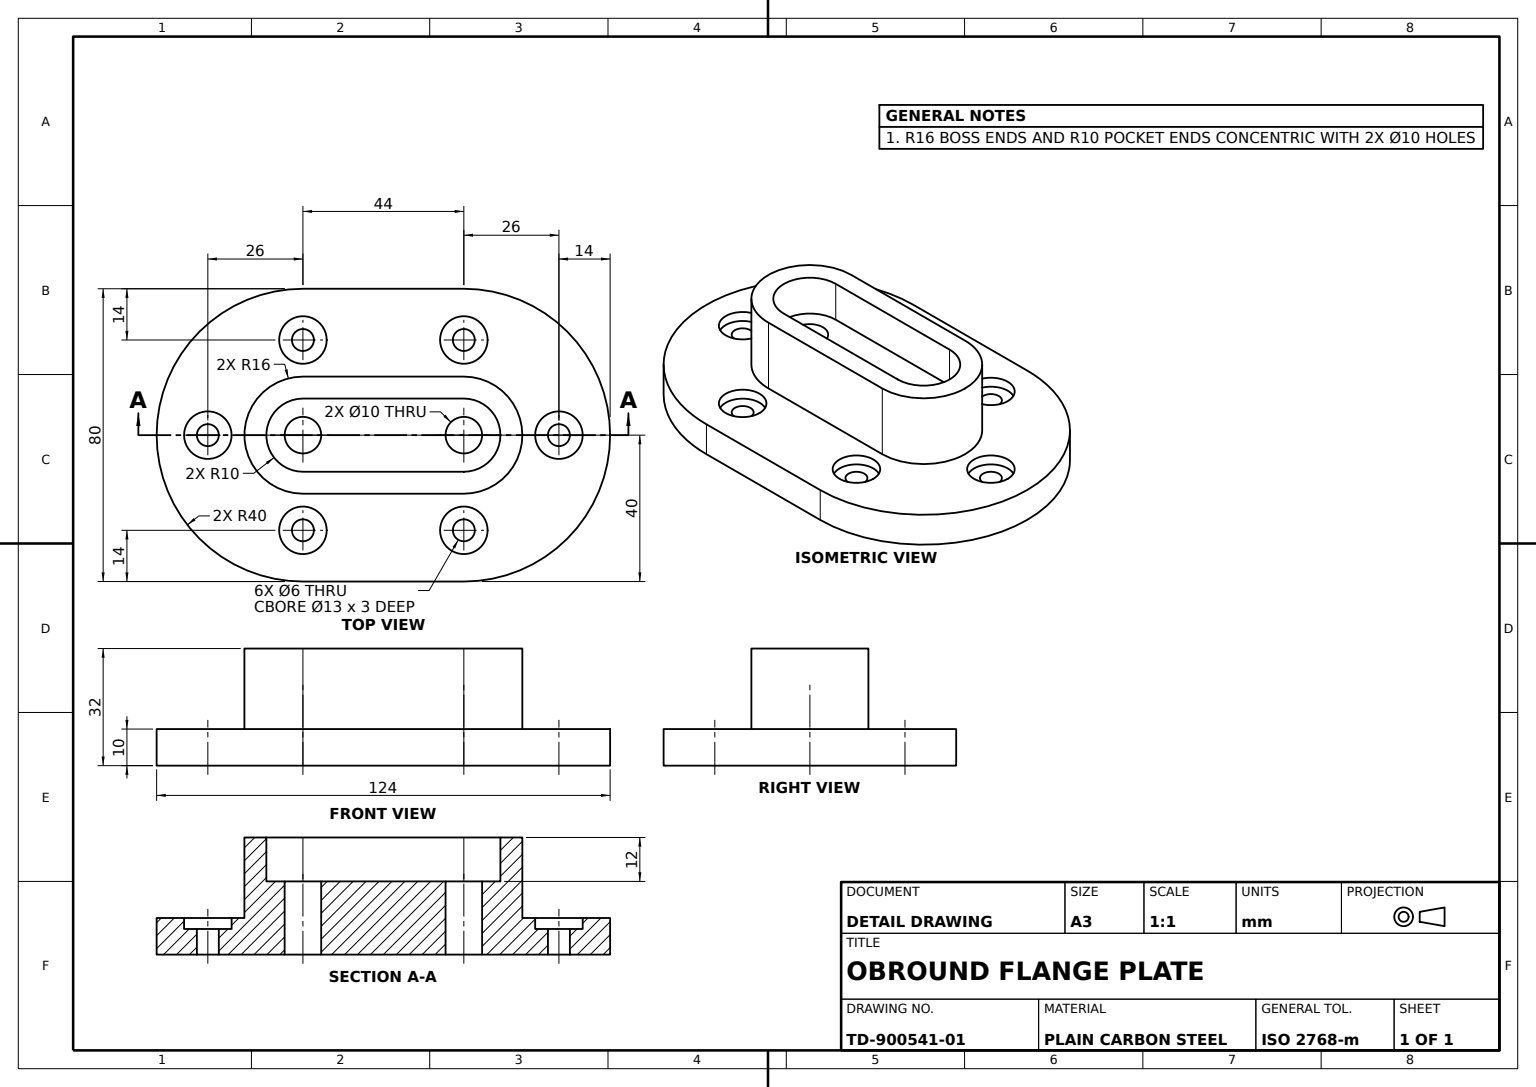
from build123d import *

# Parameters (mm, degrees)
BASE_PLATE_DEPTH        = 10
SLOT_BOSS_DEPTH         = 22
SECONDARY_BOSS_DEPTH    = 10
SLOT_CUT_SKETCH_R       = 5
SLOT_THROUGH_CUT_DEPTH  = 34.5
COUNTERBORE_SKETCH_R    = 6.5
COUNTERBORES_6X_DEPTH   = 3
MOUNTING_HOLE_SKETCH_R  = 3
MOUNTING_HOLES_6X_DEPTH = 88


with BuildPart() as part:
    # Base Plate Sketch → Base Plate (new body)
    with BuildSketch(Plane(origin=(0, 0, 0), x_dir=(1, 0, 0), z_dir=(0, 1, 0))):
        with BuildLine():
            Line((40, 22), (40, -22))
            ThreePointArc((40, -22), (0, -62), (-40, -22))
            Line((-40, -22), (-40, 22))
            ThreePointArc((-40, 22), (0, 62), (40, 22))
        make_face()
    extrude(amount=BASE_PLATE_DEPTH)

    # Slot Boss Sketch → Slot Boss (add)
    with BuildSketch(Plane(origin=(0, 10, 0), x_dir=(1, 0, 0), z_dir=(0, 1, 0))):
        with BuildLine():
            Line((16, 22), (16, -22))
            ThreePointArc((16, -22), (0, -38), (-16, -22))
            Line((-16, -22), (-16, 22))
            ThreePointArc((-16, 22), (0, 38), (16, 22))
        make_face()
        with BuildLine():
            Line((10, 22), (10, -22))
            ThreePointArc((10, -22), (0, -32), (-10, -22))
            Line((-10, -22), (-10, 22))
            ThreePointArc((-10, 22), (0, 32), (10, 22))
        make_face(mode=Mode.SUBTRACT)
    extrude(amount=SLOT_BOSS_DEPTH)

    # Secondary Boss Sketch → Secondary Boss (add)
    with BuildSketch(Plane(origin=(0, 10, 0), x_dir=(1, 0, 0), z_dir=(0, 1, 0))):
        with BuildLine():
            Line((-10, 22), (-10, -22))
            ThreePointArc((-10, -22), (0, -32), (10, -22))
            Line((10, -22), (10, 22))
            ThreePointArc((10, 22), (0, 32), (-10, 22))
        make_face()
    extrude(amount=SECONDARY_BOSS_DEPTH)

    # Slot Cut Sketch → Slot Through Cut (cut, symmetric)
    with BuildSketch(Plane(origin=(0, 10, 0), x_dir=(1, 0, 0), z_dir=(0, 1, 0))):
        with Locations(Location((0, 22, 0), (0, 0, 270))):
            Circle(SLOT_CUT_SKETCH_R)
        with Locations(Location((0, -22, 0), (0, 0, 270))):
            Circle(SLOT_CUT_SKETCH_R)
    extrude(amount=SLOT_THROUGH_CUT_DEPTH, both=True, mode=Mode.SUBTRACT)

    # Counterbore Sketch → Counterbores 6x (cut)
    with BuildSketch(Plane(origin=(0, 10, 0), x_dir=(1, 0, 0), z_dir=(0, 1, 0))):
        with Locations(Location((0, -48, 0), (0, 0, 270))):
            Circle(COUNTERBORE_SKETCH_R)
        with Locations(Location((0, 48, 0), (0, 0, 270))):
            Circle(COUNTERBORE_SKETCH_R)
        with Locations(Location((26, -22, 0), (0, 0, 270))):
            Circle(COUNTERBORE_SKETCH_R)
        with Locations(Location((-26, -22, 0), (0, 0, 270))):
            Circle(COUNTERBORE_SKETCH_R)
        with Locations(Location((26, 22, 0), (0, 0, 90))):
            Circle(COUNTERBORE_SKETCH_R)
        with Locations(Location((-26, 22, 0), (0, 0, 90))):
            Circle(COUNTERBORE_SKETCH_R)
    extrude(amount=-COUNTERBORES_6X_DEPTH, mode=Mode.SUBTRACT)

    # Mounting Hole Sketch → Mounting Holes 6x (cut)
    with BuildSketch(Plane(origin=(0, 10, 0), x_dir=(1, 0, 0), z_dir=(0, 1, 0))):
        with Locations(Location((0, -48, 0), (0, 0, 270))):
            Circle(MOUNTING_HOLE_SKETCH_R)
        with Locations(Location((26, -22, 0), (0, 0, 270))):
            Circle(MOUNTING_HOLE_SKETCH_R)
        with Locations(Location((26, 22, 0), (0, 0, 270))):
            Circle(MOUNTING_HOLE_SKETCH_R)
        with Locations(Location((0, 48, 0), (0, 0, 270))):
            Circle(MOUNTING_HOLE_SKETCH_R)
        with Locations(Location((-26, 22, 0), (0, 0, 270))):
            Circle(MOUNTING_HOLE_SKETCH_R)
        with Locations(Location((-26, -22, 0), (0, 0, 270))):
            Circle(MOUNTING_HOLE_SKETCH_R)
    extrude(amount=-MOUNTING_HOLES_6X_DEPTH, mode=Mode.SUBTRACT)


solid = part.part
